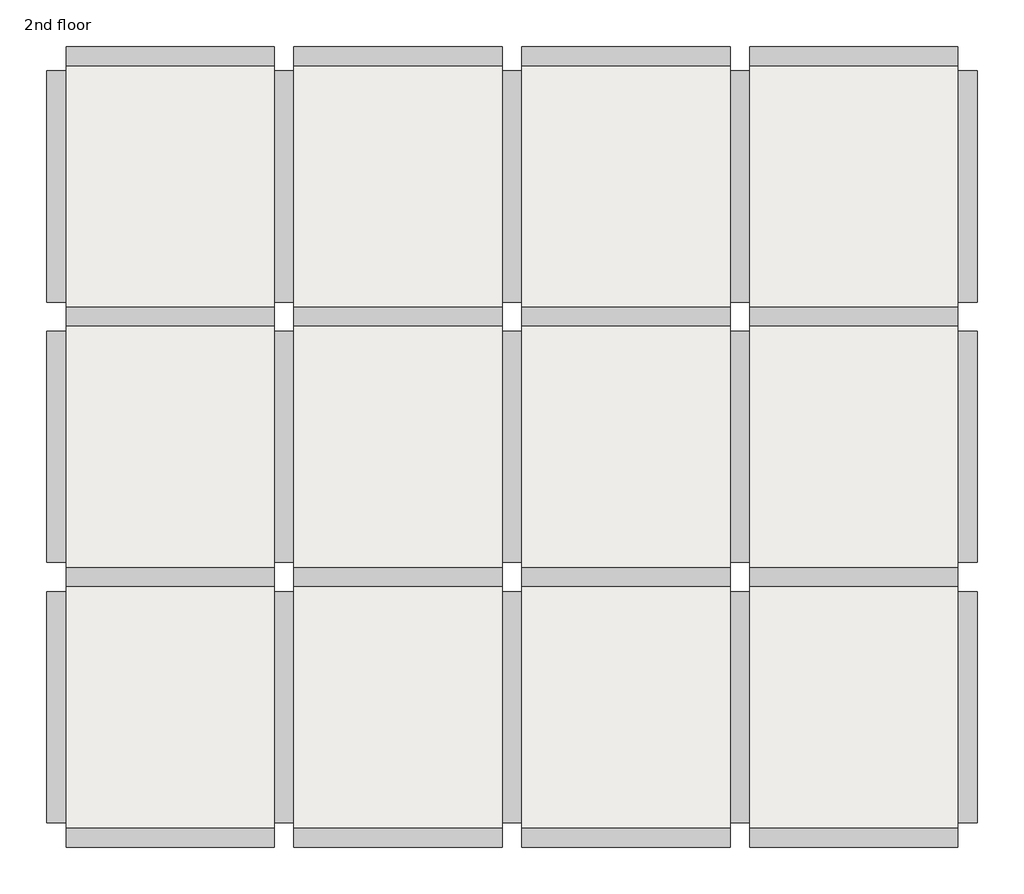
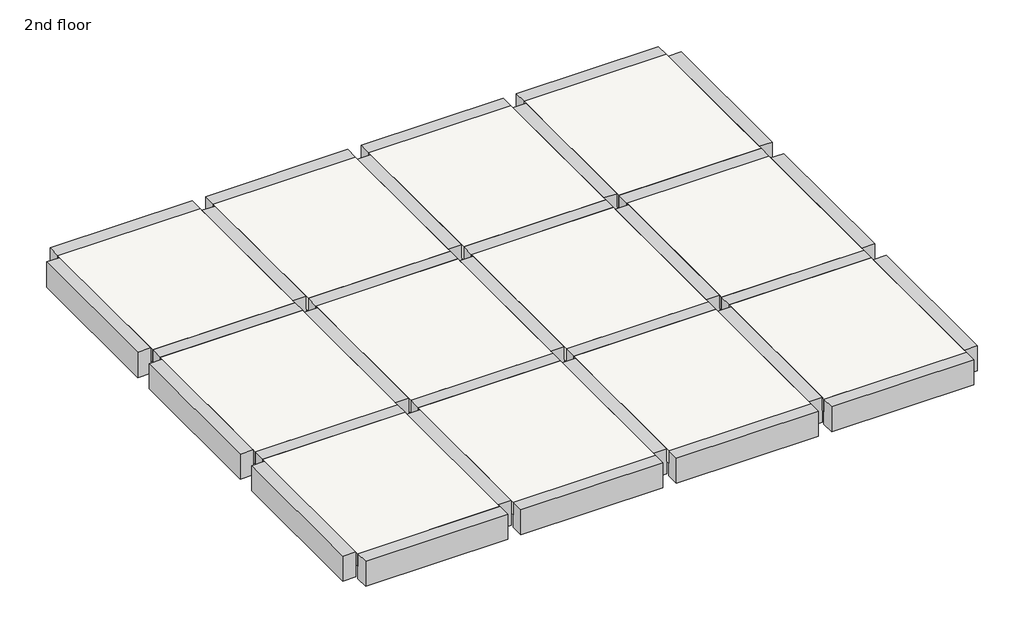
# One storey: 31 beams, 12 slabs.
"""IFC4 building model written with IfcOpenShell, lengths in millimetres."""

from ifc_helpers import new_model, si_unit, frame, origin, place, context, project, spatial, polyline, outline, extrude, faceted_brep, element, save

model = new_model("IFC4")

# Units and contexts
model_context = context("Model", 3, world=origin())
ifc_project = project(units=[si_unit("LENGTHUNIT", "METRE", prefix="MILLI")], contexts=[model_context])

# Site, building, storey
site = spatial("IfcSite", under=ifc_project)
building = spatial("IfcBuilding", under=site)
storey = spatial("IfcBuildingStorey", under=building, Name="2nd floor", Elevation=6096.0)

# Beams
placement = place(None, origin())
element("IfcBeam", 1, ObjectType="M_Concrete-Rectangular Beam : 300 x 600mm", at=placement, inside=storey, context=model_context, shape_type="SweptSolid", body=[
    extrude(outline(polyline([(-11389.0800189, 9311.4575251), (-11089.0800189, 9311.4575251), (-11089.0800189, 5761.4575251), (-11389.0800189, 5761.4575251), (-11389.0800189, 9311.4575251)])), frame((0.0, 0.0, 5496.0), z_axis=(0.0, 0.0, 1.0), x_axis=(1.0, 0.0, 0.0)), (0.0, 0.0, 1.0), 600.0),
])
element("IfcBeam", 2, ObjectType="M_Concrete-Rectangular Beam : 300 x 600mm", at=placement, inside=storey, context=model_context, shape_type="SweptSolid", body=[
    extrude(outline(polyline([(-11389.0800189, 13311.4575251), (-11089.0800189, 13311.4575251), (-11089.0800189, 9761.4575251), (-11389.0800189, 9761.4575251), (-11389.0800189, 13311.4575251)])), frame((0.0, 0.0, 5496.0), z_axis=(0.0, 0.0, 1.0), x_axis=(1.0, 0.0, 0.0)), (0.0, 0.0, 1.0), 600.0),
])
element("IfcBeam", 3, ObjectType="M_Concrete-Rectangular Beam : 300 x 600mm", at=placement, inside=storey, context=model_context, shape_type="SweptSolid", body=[
    extrude(outline(polyline([(-11389.0800189, 17311.4575251), (-11089.0800189, 17311.4575251), (-11089.0800189, 13761.4575251), (-11389.0800189, 13761.4575251), (-11389.0800189, 17311.4575251)])), frame((0.0, 0.0, 5496.0), z_axis=(0.0, 0.0, 1.0), x_axis=(1.0, 0.0, 0.0)), (0.0, 0.0, 1.0), 600.0),
])
element("IfcBeam", 4, ObjectType="M_Concrete-Rectangular Beam : 300 x 600mm", at=placement, inside=storey, context=model_context, shape_type="SweptSolid", body=[
    extrude(outline(polyline([(-7889.0800189, 9311.4575251), (-7589.0800189, 9311.4575251), (-7589.0800189, 5761.4575251), (-7889.0800189, 5761.4575251), (-7889.0800189, 9311.4575251)])), frame((0.0, 0.0, 5496.0), z_axis=(0.0, 0.0, 1.0), x_axis=(1.0, 0.0, 0.0)), (0.0, 0.0, 1.0), 600.0),
])
element("IfcBeam", 5, ObjectType="M_Concrete-Rectangular Beam : 300 x 600mm", at=placement, inside=storey, context=model_context, shape_type="SweptSolid", body=[
    extrude(outline(polyline([(-7889.0800189, 13311.4575251), (-7589.0800189, 13311.4575251), (-7589.0800189, 9761.4575251), (-7889.0800189, 9761.4575251), (-7889.0800189, 13311.4575251)])), frame((0.0, 0.0, 5496.0), z_axis=(0.0, 0.0, 1.0), x_axis=(1.0, 0.0, 0.0)), (0.0, 0.0, 1.0), 600.0),
])
element("IfcBeam", 6, ObjectType="M_Concrete-Rectangular Beam : 300 x 600mm", at=placement, inside=storey, context=model_context, shape_type="SweptSolid", body=[
    extrude(outline(polyline([(-7889.0800189, 17311.4575251), (-7589.0800189, 17311.4575251), (-7589.0800189, 13761.4575251), (-7889.0800189, 13761.4575251), (-7889.0800189, 17311.4575251)])), frame((0.0, 0.0, 5496.0), z_axis=(0.0, 0.0, 1.0), x_axis=(1.0, 0.0, 0.0)), (0.0, 0.0, 1.0), 600.0),
])
element("IfcBeam", 7, ObjectType="M_Concrete-Rectangular Beam : 300 x 600mm", at=placement, inside=storey, context=model_context, shape_type="SweptSolid", body=[
    extrude(outline(polyline([(-4389.0800189, 9311.4575251), (-4089.0800189, 9311.4575251), (-4089.0800189, 5761.4575251), (-4389.0800189, 5761.4575251), (-4389.0800189, 9311.4575251)])), frame((0.0, 0.0, 5496.0), z_axis=(0.0, 0.0, 1.0), x_axis=(1.0, 0.0, 0.0)), (0.0, 0.0, 1.0), 600.0),
])
element("IfcBeam", 8, ObjectType="M_Concrete-Rectangular Beam : 300 x 600mm", at=placement, inside=storey, context=model_context, shape_type="SweptSolid", body=[
    extrude(outline(polyline([(-4389.0800189, 13311.4575251), (-4089.0800189, 13311.4575251), (-4089.0800189, 9761.4575251), (-4389.0800189, 9761.4575251), (-4389.0800189, 13311.4575251)])), frame((0.0, 0.0, 5496.0), z_axis=(0.0, 0.0, 1.0), x_axis=(1.0, 0.0, 0.0)), (0.0, 0.0, 1.0), 600.0),
])
element("IfcBeam", 9, ObjectType="M_Concrete-Rectangular Beam : 300 x 600mm", at=placement, inside=storey, context=model_context, shape_type="SweptSolid", body=[
    extrude(outline(polyline([(-4389.0800189, 17311.4575251), (-4089.0800189, 17311.4575251), (-4089.0800189, 13761.4575251), (-4389.0800189, 13761.4575251), (-4389.0800189, 17311.4575251)])), frame((0.0, 0.0, 5496.0), z_axis=(0.0, 0.0, 1.0), x_axis=(1.0, 0.0, 0.0)), (0.0, 0.0, 1.0), 600.0),
])
element("IfcBeam", 10, ObjectType="M_Concrete-Rectangular Beam : 300 x 600mm", at=placement, inside=storey, context=model_context, shape_type="SweptSolid", body=[
    extrude(outline(polyline([(-889.0800189, 9311.4575251), (-589.0800189, 9311.4575251), (-589.0800189, 5761.4575251), (-889.0800189, 5761.4575251), (-889.0800189, 9311.4575251)])), frame((0.0, 0.0, 5496.0), z_axis=(0.0, 0.0, 1.0), x_axis=(1.0, 0.0, 0.0)), (0.0, 0.0, 1.0), 600.0),
])
element("IfcBeam", 11, ObjectType="M_Concrete-Rectangular Beam : 300 x 600mm", at=placement, inside=storey, context=model_context, shape_type="SweptSolid", body=[
    extrude(outline(polyline([(-889.0800189, 13311.4575251), (-589.0800189, 13311.4575251), (-589.0800189, 9761.4575251), (-889.0800189, 9761.4575251), (-889.0800189, 13311.4575251)])), frame((0.0, 0.0, 5496.0), z_axis=(0.0, 0.0, 1.0), x_axis=(1.0, 0.0, 0.0)), (0.0, 0.0, 1.0), 600.0),
])
element("IfcBeam", 12, ObjectType="M_Concrete-Rectangular Beam : 300 x 600mm", at=placement, inside=storey, context=model_context, shape_type="SweptSolid", body=[
    extrude(outline(polyline([(-889.0800189, 17311.4575251), (-589.0800189, 17311.4575251), (-589.0800189, 13761.4575251), (-889.0800189, 13761.4575251), (-889.0800189, 17311.4575251)])), frame((0.0, 0.0, 5496.0), z_axis=(0.0, 0.0, 1.0), x_axis=(1.0, 0.0, 0.0)), (0.0, 0.0, 1.0), 600.0),
])
element("IfcBeam", 13, ObjectType="M_Concrete-Rectangular Beam : 300 x 600mm", at=placement, inside=storey, context=model_context, shape_type="SweptSolid", body=[
    extrude(outline(polyline([(2610.9199811, 9311.4575251), (2910.9199811, 9311.4575251), (2910.9199811, 5761.4575251), (2610.9199811, 5761.4575251), (2610.9199811, 9311.4575251)])), frame((0.0, 0.0, 5496.0), z_axis=(0.0, 0.0, 1.0), x_axis=(1.0, 0.0, 0.0)), (0.0, 0.0, 1.0), 600.0),
])
element("IfcBeam", 14, ObjectType="M_Concrete-Rectangular Beam : 300 x 600mm", at=placement, inside=storey, context=model_context, shape_type="SweptSolid", body=[
    extrude(outline(polyline([(2610.9199811, 13311.4575251), (2910.9199811, 13311.4575251), (2910.9199811, 9761.4575251), (2610.9199811, 9761.4575251), (2610.9199811, 13311.4575251)])), frame((0.0, 0.0, 5496.0), z_axis=(0.0, 0.0, 1.0), x_axis=(1.0, 0.0, 0.0)), (0.0, 0.0, 1.0), 600.0),
])
element("IfcBeam", 15, ObjectType="M_Concrete-Rectangular Beam : 300 x 600mm", at=placement, inside=storey, context=model_context, shape_type="SweptSolid", body=[
    extrude(outline(polyline([(2610.9199811, 17311.4575251), (2910.9199811, 17311.4575251), (2910.9199811, 13761.4575251), (2610.9199811, 13761.4575251), (2610.9199811, 17311.4575251)])), frame((0.0, 0.0, 5496.0), z_axis=(0.0, 0.0, 1.0), x_axis=(1.0, 0.0, 0.0)), (0.0, 0.0, 1.0), 600.0),
])
element("IfcBeam", 16, ObjectType="M_Concrete-Rectangular Beam : 300 x 600mm", at=placement, inside=storey, context=model_context, shape_type="Brep", body=[
    faceted_brep([(-11089.0800189, 17386.4575251, 6096.0), (-7889.0800189, 17386.4575251, 6096.0), (-7889.0800189, 17686.4575251, 6096.0), (-11089.0800189, 17686.4575251, 6096.0), (-11089.0800189, 17386.4575251, 5796.0), (-11089.0800189, 17386.4575251, 5496.0), (-7889.0800189, 17386.4575251, 5496.0), (-7889.0800189, 17386.4575251, 5796.0), (-7889.0800189, 17686.4575251, 5496.0), (-11089.0800189, 17686.4575251, 5496.0)], [[[0, 1, 2, 3]], [[0, 4, 5, 6, 7, 1]], [[8, 6, 5, 9]], [[9, 3, 2, 8]], [[5, 4, 0, 3, 9]], [[1, 7, 6, 8, 2]]]),
])
element("IfcBeam", 17, ObjectType="M_Concrete-Rectangular Beam : 300 x 600mm", at=placement, inside=storey, context=model_context, shape_type="Brep", body=[
    faceted_brep([(-7589.0800189, 17386.4575251, 6096.0), (-4389.0800189, 17386.4575251, 6096.0), (-4389.0800189, 17686.4575251, 6096.0), (-7589.0800189, 17686.4575251, 6096.0), (-7589.0800189, 17386.4575251, 5796.0), (-7589.0800189, 17386.4575251, 5496.0), (-4389.0800189, 17386.4575251, 5496.0), (-4389.0800189, 17386.4575251, 5796.0), (-4389.0800189, 17686.4575251, 5496.0), (-7589.0800189, 17686.4575251, 5496.0)], [[[0, 1, 2, 3]], [[0, 4, 5, 6, 7, 1]], [[8, 6, 5, 9]], [[9, 3, 2, 8]], [[5, 4, 0, 3, 9]], [[1, 7, 6, 8, 2]]]),
])
element("IfcBeam", 18, ObjectType="M_Concrete-Rectangular Beam : 300 x 600mm", at=placement, inside=storey, context=model_context, shape_type="Brep", body=[
    faceted_brep([(-4089.0800189, 17386.4575251, 6096.0), (-889.0800189, 17386.4575251, 6096.0), (-889.0800189, 17686.4575251, 6096.0), (-4089.0800189, 17686.4575251, 6096.0), (-4089.0800189, 17386.4575251, 5796.0), (-4089.0800189, 17386.4575251, 5496.0), (-889.0800189, 17386.4575251, 5496.0), (-889.0800189, 17386.4575251, 5796.0), (-889.0800189, 17686.4575251, 5496.0), (-4089.0800189, 17686.4575251, 5496.0)], [[[0, 1, 2, 3]], [[0, 4, 5, 6, 7, 1]], [[8, 6, 5, 9]], [[9, 3, 2, 8]], [[5, 4, 0, 3, 9]], [[1, 7, 6, 8, 2]]]),
])
element("IfcBeam", 19, ObjectType="M_Concrete-Rectangular Beam : 300 x 600mm", at=placement, inside=storey, context=model_context, shape_type="Brep", body=[
    faceted_brep([(-589.0800189, 17386.4575251, 6096.0), (2610.9199811, 17386.4575251, 6096.0), (2610.9199811, 17686.4575251, 6096.0), (-589.0800189, 17686.4575251, 6096.0), (-589.0800189, 17386.4575251, 5796.0), (-589.0800189, 17386.4575251, 5496.0), (2610.9199811, 17386.4575251, 5496.0), (2610.9199811, 17386.4575251, 5796.0), (2610.9199811, 17686.4575251, 5496.0), (-589.0800189, 17686.4575251, 5496.0)], [[[0, 1, 2, 3]], [[0, 4, 5, 6, 7, 1]], [[8, 6, 5, 9]], [[9, 3, 2, 8]], [[5, 4, 0, 3, 9]], [[1, 7, 6, 8, 2]]]),
])
element("IfcBeam", 20, ObjectType="M_Concrete-Rectangular Beam : 300 x 600mm", at=placement, inside=storey, context=model_context, shape_type="Brep", body=[
    faceted_brep([(-11089.0800189, 13386.4575251, 6096.0), (-7889.0800189, 13386.4575251, 6096.0), (-7889.0800189, 13686.4575251, 6096.0), (-11089.0800189, 13686.4575251, 6096.0), (-11089.0800189, 13386.4575251, 5796.0), (-11089.0800189, 13386.4575251, 5496.0), (-7889.0800189, 13386.4575251, 5496.0), (-7889.0800189, 13386.4575251, 5796.0), (-7889.0800189, 13686.4575251, 5496.0), (-11089.0800189, 13686.4575251, 5496.0), (-11089.0800189, 13686.4575251, 5796.0), (-7889.0800189, 13686.4575251, 5796.0)], [[[0, 1, 2, 3]], [[0, 4, 5, 6, 7, 1]], [[8, 6, 5, 9]], [[9, 10, 3, 2, 11, 8]], [[5, 4, 0, 3, 10, 9]], [[1, 7, 6, 8, 11, 2]]]),
])
element("IfcBeam", 21, ObjectType="M_Concrete-Rectangular Beam : 300 x 600mm", at=placement, inside=storey, context=model_context, shape_type="Brep", body=[
    faceted_brep([(-7589.0800189, 13686.4575251, 6096.0), (-7589.0800189, 13386.4575251, 6096.0), (-4389.0800189, 13386.4575251, 6096.0), (-4389.0800189, 13686.4575251, 6096.0), (-7589.0800189, 13386.4575251, 5796.0), (-7589.0800189, 13386.4575251, 5496.0), (-4389.0800189, 13386.4575251, 5496.0), (-4389.0800189, 13386.4575251, 5796.0), (-7589.0800189, 13686.4575251, 5496.0), (-4389.0800189, 13686.4575251, 5496.0), (-7589.0800189, 13686.4575251, 5796.0), (-4389.0800189, 13686.4575251, 5796.0)], [[[0, 1, 2, 3]], [[1, 4, 5, 6, 7, 2]], [[5, 8, 9, 6]], [[8, 10, 0, 3, 11, 9]], [[5, 4, 1, 0, 10, 8]], [[2, 7, 6, 9, 11, 3]]]),
])
element("IfcBeam", 22, ObjectType="M_Concrete-Rectangular Beam : 300 x 600mm", at=placement, inside=storey, context=model_context, shape_type="Brep", body=[
    faceted_brep([(-4089.0800189, 13686.4575251, 6096.0), (-4089.0800189, 13386.4575251, 6096.0), (-889.0800189, 13386.4575251, 6096.0), (-889.0800189, 13686.4575251, 6096.0), (-4089.0800189, 13386.4575251, 5796.0), (-4089.0800189, 13386.4575251, 5496.0), (-889.0800189, 13386.4575251, 5496.0), (-889.0800189, 13386.4575251, 5796.0), (-4089.0800189, 13686.4575251, 5496.0), (-889.0800189, 13686.4575251, 5496.0), (-4089.0800189, 13686.4575251, 5796.0), (-889.0800189, 13686.4575251, 5796.0)], [[[0, 1, 2, 3]], [[1, 4, 5, 6, 7, 2]], [[5, 8, 9, 6]], [[8, 10, 0, 3, 11, 9]], [[5, 4, 1, 0, 10, 8]], [[2, 7, 6, 9, 11, 3]]]),
])
element("IfcBeam", 23, ObjectType="M_Concrete-Rectangular Beam : 300 x 600mm", at=placement, inside=storey, context=model_context, shape_type="Brep", body=[
    faceted_brep([(-589.0800189, 13686.4575251, 6096.0), (-589.0800189, 13386.4575251, 6096.0), (2610.9199811, 13386.4575251, 6096.0), (2610.9199811, 13686.4575251, 6096.0), (-589.0800189, 13386.4575251, 5796.0), (-589.0800189, 13386.4575251, 5496.0), (2610.9199811, 13386.4575251, 5496.0), (2610.9199811, 13386.4575251, 5796.0), (-589.0800189, 13686.4575251, 5496.0), (2610.9199811, 13686.4575251, 5496.0), (-589.0800189, 13686.4575251, 5796.0), (2610.9199811, 13686.4575251, 5796.0)], [[[0, 1, 2, 3]], [[1, 4, 5, 6, 7, 2]], [[5, 8, 9, 6]], [[8, 10, 0, 3, 11, 9]], [[5, 4, 1, 0, 10, 8]], [[2, 7, 6, 9, 11, 3]]]),
])
element("IfcBeam", 24, ObjectType="M_Concrete-Rectangular Beam : 300 x 600mm", at=placement, inside=storey, context=model_context, shape_type="Brep", body=[
    faceted_brep([(-11089.0800189, 9386.4575251, 6096.0), (-7889.0800189, 9386.4575251, 6096.0), (-7889.0800189, 9686.4575251, 6096.0), (-11089.0800189, 9686.4575251, 6096.0), (-11089.0800189, 9386.4575251, 5796.0), (-11089.0800189, 9386.4575251, 5496.0), (-7889.0800189, 9386.4575251, 5496.0), (-7889.0800189, 9386.4575251, 5796.0), (-7889.0800189, 9686.4575251, 5496.0), (-11089.0800189, 9686.4575251, 5496.0), (-11089.0800189, 9686.4575251, 5796.0), (-7889.0800189, 9686.4575251, 5796.0)], [[[0, 1, 2, 3]], [[0, 4, 5, 6, 7, 1]], [[8, 6, 5, 9]], [[9, 10, 3, 2, 11, 8]], [[5, 4, 0, 3, 10, 9]], [[1, 7, 6, 8, 11, 2]]]),
])
element("IfcBeam", 25, ObjectType="M_Concrete-Rectangular Beam : 300 x 600mm", at=placement, inside=storey, context=model_context, shape_type="Brep", body=[
    faceted_brep([(-7589.0800189, 9686.4575251, 6096.0), (-7589.0800189, 9386.4575251, 6096.0), (-4389.0800189, 9386.4575251, 6096.0), (-4389.0800189, 9686.4575251, 6096.0), (-7589.0800189, 9386.4575251, 5796.0), (-7589.0800189, 9386.4575251, 5496.0), (-4389.0800189, 9386.4575251, 5496.0), (-4389.0800189, 9386.4575251, 5796.0), (-7589.0800189, 9686.4575251, 5496.0), (-4389.0800189, 9686.4575251, 5496.0), (-7589.0800189, 9686.4575251, 5796.0), (-4389.0800189, 9686.4575251, 5796.0)], [[[0, 1, 2, 3]], [[1, 4, 5, 6, 7, 2]], [[5, 8, 9, 6]], [[8, 10, 0, 3, 11, 9]], [[5, 4, 1, 0, 10, 8]], [[2, 7, 6, 9, 11, 3]]]),
])
element("IfcBeam", 26, ObjectType="M_Concrete-Rectangular Beam : 300 x 600mm", at=placement, inside=storey, context=model_context, shape_type="Brep", body=[
    faceted_brep([(-4089.0800189, 9686.4575251, 6096.0), (-4089.0800189, 9386.4575251, 6096.0), (-889.0800189, 9386.4575251, 6096.0), (-889.0800189, 9686.4575251, 6096.0), (-4089.0800189, 9386.4575251, 5796.0), (-4089.0800189, 9386.4575251, 5496.0), (-889.0800189, 9386.4575251, 5496.0), (-889.0800189, 9386.4575251, 5796.0), (-4089.0800189, 9686.4575251, 5496.0), (-889.0800189, 9686.4575251, 5496.0), (-4089.0800189, 9686.4575251, 5796.0), (-889.0800189, 9686.4575251, 5796.0)], [[[0, 1, 2, 3]], [[1, 4, 5, 6, 7, 2]], [[5, 8, 9, 6]], [[8, 10, 0, 3, 11, 9]], [[5, 4, 1, 0, 10, 8]], [[2, 7, 6, 9, 11, 3]]]),
])
element("IfcBeam", 27, ObjectType="M_Concrete-Rectangular Beam : 300 x 600mm", at=placement, inside=storey, context=model_context, shape_type="Brep", body=[
    faceted_brep([(-589.0800189, 9686.4575251, 6096.0), (-589.0800189, 9386.4575251, 6096.0), (2610.9199811, 9386.4575251, 6096.0), (2610.9199811, 9686.4575251, 6096.0), (-589.0800189, 9386.4575251, 5796.0), (-589.0800189, 9386.4575251, 5496.0), (2610.9199811, 9386.4575251, 5496.0), (2610.9199811, 9386.4575251, 5796.0), (-589.0800189, 9686.4575251, 5496.0), (2610.9199811, 9686.4575251, 5496.0), (-589.0800189, 9686.4575251, 5796.0), (2610.9199811, 9686.4575251, 5796.0)], [[[0, 1, 2, 3]], [[1, 4, 5, 6, 7, 2]], [[5, 8, 9, 6]], [[8, 10, 0, 3, 11, 9]], [[5, 4, 1, 0, 10, 8]], [[2, 7, 6, 9, 11, 3]]]),
])
element("IfcBeam", 28, ObjectType="M_Concrete-Rectangular Beam : 300 x 600mm", at=placement, inside=storey, context=model_context, shape_type="Brep", body=[
    faceted_brep([(-7889.0800189, 5386.4575251, 6096.0), (-7889.0800189, 5686.4575251, 6096.0), (-11089.0800189, 5686.4575251, 6096.0), (-11089.0800189, 5386.4575251, 6096.0), (-11089.0800189, 5386.4575251, 5496.0), (-7889.0800189, 5386.4575251, 5496.0), (-11089.0800189, 5686.4575251, 5496.0), (-7889.0800189, 5686.4575251, 5496.0), (-11089.0800189, 5686.4575251, 5796.0), (-7889.0800189, 5686.4575251, 5796.0)], [[[0, 1, 2, 3]], [[3, 4, 5, 0]], [[6, 7, 5, 4]], [[6, 8, 2, 1, 9, 7]], [[2, 8, 6, 4, 3]], [[0, 5, 7, 9, 1]]]),
])
element("IfcBeam", 29, ObjectType="M_Concrete-Rectangular Beam : 300 x 600mm", at=placement, inside=storey, context=model_context, shape_type="Brep", body=[
    faceted_brep([(-4389.0800189, 5386.4575251, 6096.0), (-4389.0800189, 5686.4575251, 6096.0), (-7589.0800189, 5686.4575251, 6096.0), (-7589.0800189, 5386.4575251, 6096.0), (-7589.0800189, 5386.4575251, 5496.0), (-4389.0800189, 5386.4575251, 5496.0), (-7589.0800189, 5686.4575251, 5496.0), (-4389.0800189, 5686.4575251, 5496.0), (-7589.0800189, 5686.4575251, 5796.0), (-4389.0800189, 5686.4575251, 5796.0)], [[[0, 1, 2, 3]], [[3, 4, 5, 0]], [[6, 7, 5, 4]], [[6, 8, 2, 1, 9, 7]], [[2, 8, 6, 4, 3]], [[0, 5, 7, 9, 1]]]),
])
element("IfcBeam", 30, ObjectType="M_Concrete-Rectangular Beam : 300 x 600mm", at=placement, inside=storey, context=model_context, shape_type="Brep", body=[
    faceted_brep([(-889.0800189, 5386.4575251, 6096.0), (-889.0800189, 5686.4575251, 6096.0), (-4089.0800189, 5686.4575251, 6096.0), (-4089.0800189, 5386.4575251, 6096.0), (-4089.0800189, 5386.4575251, 5496.0), (-889.0800189, 5386.4575251, 5496.0), (-4089.0800189, 5686.4575251, 5496.0), (-889.0800189, 5686.4575251, 5496.0), (-4089.0800189, 5686.4575251, 5796.0), (-889.0800189, 5686.4575251, 5796.0)], [[[0, 1, 2, 3]], [[3, 4, 5, 0]], [[6, 7, 5, 4]], [[6, 8, 2, 1, 9, 7]], [[2, 8, 6, 4, 3]], [[0, 5, 7, 9, 1]]]),
])
element("IfcBeam", 31, ObjectType="M_Concrete-Rectangular Beam : 300 x 600mm", at=placement, inside=storey, context=model_context, shape_type="Brep", body=[
    faceted_brep([(2610.9199811, 5386.4575251, 6096.0), (2610.9199811, 5686.4575251, 6096.0), (-589.0800189, 5686.4575251, 6096.0), (-589.0800189, 5386.4575251, 6096.0), (-589.0800189, 5386.4575251, 5496.0), (2610.9199811, 5386.4575251, 5496.0), (-589.0800189, 5686.4575251, 5496.0), (2610.9199811, 5686.4575251, 5496.0), (-589.0800189, 5686.4575251, 5796.0), (2610.9199811, 5686.4575251, 5796.0)], [[[0, 1, 2, 3]], [[3, 4, 5, 0]], [[6, 7, 5, 4]], [[6, 8, 2, 1, 9, 7]], [[2, 8, 6, 4, 3]], [[0, 5, 7, 9, 1]]]),
])

# Slabs
element("IfcSlab", 32, ObjectType="Generic 300mm", at=placement, inside=storey, context=model_context, shape_type="Brep", body=[
    faceted_brep([(-7889.0800189, 17386.4575251, 5796.0), (-7889.0800189, 13686.4575251, 5796.0), (-11089.0800189, 13686.4575251, 5796.0), (-11089.0800189, 17386.4575251, 5796.0), (-7889.0800189, 17386.4575251, 6096.0), (-11089.0800189, 17386.4575251, 6096.0), (-11089.0800189, 17311.4575251, 6096.0), (-11089.0800189, 13761.4575251, 6096.0), (-11089.0800189, 13686.4575251, 6096.0), (-7889.0800189, 13686.4575251, 6096.0), (-7889.0800189, 13761.4575251, 6096.0), (-7889.0800189, 17311.4575251, 6096.0)], [[[0, 1, 2, 3]], [[4, 5, 6, 7, 8, 9, 10, 11]], [[1, 0, 4, 11, 10, 9]], [[2, 1, 9, 8]], [[3, 2, 8, 7, 6, 5]], [[0, 3, 5, 4]]]),
])
element("IfcSlab", 33, ObjectType="Generic 300mm", at=placement, inside=storey, context=model_context, shape_type="Brep", body=[
    faceted_brep([(-4389.0800189, 17386.4575251, 5796.0), (-4389.0800189, 13686.4575251, 5796.0), (-7589.0800189, 13686.4575251, 5796.0), (-7589.0800189, 17386.4575251, 5796.0), (-4389.0800189, 17386.4575251, 6096.0), (-7589.0800189, 17386.4575251, 6096.0), (-7589.0800189, 17311.4575251, 6096.0), (-7589.0800189, 13761.4575251, 6096.0), (-7589.0800189, 13686.4575251, 6096.0), (-4389.0800189, 13686.4575251, 6096.0), (-4389.0800189, 13761.4575251, 6096.0), (-4389.0800189, 17311.4575251, 6096.0)], [[[0, 1, 2, 3]], [[4, 5, 6, 7, 8, 9, 10, 11]], [[1, 0, 4, 11, 10, 9]], [[2, 1, 9, 8]], [[3, 2, 8, 7, 6, 5]], [[0, 3, 5, 4]]]),
])
element("IfcSlab", 34, ObjectType="Generic 300mm", at=placement, inside=storey, context=model_context, shape_type="Brep", body=[
    faceted_brep([(-889.0800189, 17386.4575251, 5796.0), (-889.0800189, 13686.4575251, 5796.0), (-4089.0800189, 13686.4575251, 5796.0), (-4089.0800189, 17386.4575251, 5796.0), (-889.0800189, 17386.4575251, 6096.0), (-4089.0800189, 17386.4575251, 6096.0), (-4089.0800189, 17311.4575251, 6096.0), (-4089.0800189, 13761.4575251, 6096.0), (-4089.0800189, 13686.4575251, 6096.0), (-889.0800189, 13686.4575251, 6096.0), (-889.0800189, 13761.4575251, 6096.0), (-889.0800189, 17311.4575251, 6096.0)], [[[0, 1, 2, 3]], [[4, 5, 6, 7, 8, 9, 10, 11]], [[1, 0, 4, 11, 10, 9]], [[2, 1, 9, 8]], [[3, 2, 8, 7, 6, 5]], [[0, 3, 5, 4]]]),
])
element("IfcSlab", 35, ObjectType="Generic 300mm", at=placement, inside=storey, context=model_context, shape_type="Brep", body=[
    faceted_brep([(2610.9199811, 17386.4575251, 5796.0), (2610.9199811, 13686.4575251, 5796.0), (-589.0800189, 13686.4575251, 5796.0), (-589.0800189, 17386.4575251, 5796.0), (2610.9199811, 17386.4575251, 6096.0), (-589.0800189, 17386.4575251, 6096.0), (-589.0800189, 17311.4575251, 6096.0), (-589.0800189, 13761.4575251, 6096.0), (-589.0800189, 13686.4575251, 6096.0), (2610.9199811, 13686.4575251, 6096.0), (2610.9199811, 13761.4575251, 6096.0), (2610.9199811, 17311.4575251, 6096.0)], [[[0, 1, 2, 3]], [[4, 5, 6, 7, 8, 9, 10, 11]], [[1, 0, 4, 11, 10, 9]], [[2, 1, 9, 8]], [[3, 2, 8, 7, 6, 5]], [[0, 3, 5, 4]]]),
])
element("IfcSlab", 36, ObjectType="Generic 300mm", at=placement, inside=storey, context=model_context, shape_type="Brep", body=[
    faceted_brep([(2610.9199811, 13386.4575251, 5796.0), (2610.9199811, 9686.4575251, 5796.0), (-589.0800189, 9686.4575251, 5796.0), (-589.0800189, 13386.4575251, 5796.0), (2610.9199811, 13386.4575251, 6096.0), (-589.0800189, 13386.4575251, 6096.0), (-589.0800189, 13311.4575251, 6096.0), (-589.0800189, 9761.4575251, 6096.0), (-589.0800189, 9686.4575251, 6096.0), (2610.9199811, 9686.4575251, 6096.0), (2610.9199811, 9761.4575251, 6096.0), (2610.9199811, 13311.4575251, 6096.0)], [[[0, 1, 2, 3]], [[4, 5, 6, 7, 8, 9, 10, 11]], [[1, 0, 4, 11, 10, 9]], [[2, 1, 9, 8]], [[3, 2, 8, 7, 6, 5]], [[0, 3, 5, 4]]]),
])
element("IfcSlab", 37, ObjectType="Generic 300mm", at=placement, inside=storey, context=model_context, shape_type="Brep", body=[
    faceted_brep([(2610.9199811, 9386.4575251, 5796.0), (2610.9199811, 5686.4575251, 5796.0), (-589.0800189, 5686.4575251, 5796.0), (-589.0800189, 9386.4575251, 5796.0), (2610.9199811, 9386.4575251, 6096.0), (-589.0800189, 9386.4575251, 6096.0), (-589.0800189, 9311.4575251, 6096.0), (-589.0800189, 5761.4575251, 6096.0), (-589.0800189, 5686.4575251, 6096.0), (2610.9199811, 5686.4575251, 6096.0), (2610.9199811, 5761.4575251, 6096.0), (2610.9199811, 9311.4575251, 6096.0)], [[[0, 1, 2, 3]], [[4, 5, 6, 7, 8, 9, 10, 11]], [[1, 0, 4, 11, 10, 9]], [[2, 1, 9, 8]], [[3, 2, 8, 7, 6, 5]], [[0, 3, 5, 4]]]),
])
element("IfcSlab", 38, ObjectType="Generic 300mm", at=placement, inside=storey, context=model_context, shape_type="Brep", body=[
    faceted_brep([(-889.0800189, 9386.4575251, 5796.0), (-889.0800189, 5686.4575251, 5796.0), (-4089.0800189, 5686.4575251, 5796.0), (-4089.0800189, 9386.4575251, 5796.0), (-889.0800189, 9386.4575251, 6096.0), (-4089.0800189, 9386.4575251, 6096.0), (-4089.0800189, 9311.4575251, 6096.0), (-4089.0800189, 5761.4575251, 6096.0), (-4089.0800189, 5686.4575251, 6096.0), (-889.0800189, 5686.4575251, 6096.0), (-889.0800189, 5761.4575251, 6096.0), (-889.0800189, 9311.4575251, 6096.0)], [[[0, 1, 2, 3]], [[4, 5, 6, 7, 8, 9, 10, 11]], [[1, 0, 4, 11, 10, 9]], [[2, 1, 9, 8]], [[3, 2, 8, 7, 6, 5]], [[0, 3, 5, 4]]]),
])
element("IfcSlab", 39, ObjectType="Generic 300mm", at=placement, inside=storey, context=model_context, shape_type="Brep", body=[
    faceted_brep([(-4389.0800189, 9386.4575251, 5796.0), (-4389.0800189, 5686.4575251, 5796.0), (-7589.0800189, 5686.4575251, 5796.0), (-7589.0800189, 9386.4575251, 5796.0), (-4389.0800189, 9386.4575251, 6096.0), (-7589.0800189, 9386.4575251, 6096.0), (-7589.0800189, 9311.4575251, 6096.0), (-7589.0800189, 5761.4575251, 6096.0), (-7589.0800189, 5686.4575251, 6096.0), (-4389.0800189, 5686.4575251, 6096.0), (-4389.0800189, 5761.4575251, 6096.0), (-4389.0800189, 9311.4575251, 6096.0)], [[[0, 1, 2, 3]], [[4, 5, 6, 7, 8, 9, 10, 11]], [[1, 0, 4, 11, 10, 9]], [[2, 1, 9, 8]], [[3, 2, 8, 7, 6, 5]], [[0, 3, 5, 4]]]),
])
element("IfcSlab", 40, ObjectType="Generic 300mm", at=placement, inside=storey, context=model_context, shape_type="Brep", body=[
    faceted_brep([(-7889.0800189, 9386.4575251, 5796.0), (-7889.0800189, 5686.4575251, 5796.0), (-11089.0800189, 5686.4575251, 5796.0), (-11089.0800189, 9386.4575251, 5796.0), (-7889.0800189, 9386.4575251, 6096.0), (-11089.0800189, 9386.4575251, 6096.0), (-11089.0800189, 9311.4575251, 6096.0), (-11089.0800189, 5761.4575251, 6096.0), (-11089.0800189, 5686.4575251, 6096.0), (-7889.0800189, 5686.4575251, 6096.0), (-7889.0800189, 5761.4575251, 6096.0), (-7889.0800189, 9311.4575251, 6096.0)], [[[0, 1, 2, 3]], [[4, 5, 6, 7, 8, 9, 10, 11]], [[1, 0, 4, 11, 10, 9]], [[2, 1, 9, 8]], [[3, 2, 8, 7, 6, 5]], [[0, 3, 5, 4]]]),
])
element("IfcSlab", 41, ObjectType="Generic 300mm", at=placement, inside=storey, context=model_context, shape_type="Brep", body=[
    faceted_brep([(-7889.0800189, 13386.4575251, 5796.0), (-7889.0800189, 9686.4575251, 5796.0), (-11089.0800189, 9686.4575251, 5796.0), (-11089.0800189, 13386.4575251, 5796.0), (-7889.0800189, 13386.4575251, 6096.0), (-11089.0800189, 13386.4575251, 6096.0), (-11089.0800189, 13311.4575251, 6096.0), (-11089.0800189, 9761.4575251, 6096.0), (-11089.0800189, 9686.4575251, 6096.0), (-7889.0800189, 9686.4575251, 6096.0), (-7889.0800189, 9761.4575251, 6096.0), (-7889.0800189, 13311.4575251, 6096.0)], [[[0, 1, 2, 3]], [[4, 5, 6, 7, 8, 9, 10, 11]], [[1, 0, 4, 11, 10, 9]], [[2, 1, 9, 8]], [[3, 2, 8, 7, 6, 5]], [[0, 3, 5, 4]]]),
])
element("IfcSlab", 42, ObjectType="Generic 300mm", at=placement, inside=storey, context=model_context, shape_type="Brep", body=[
    faceted_brep([(-4389.0800189, 13386.4575251, 5796.0), (-4389.0800189, 9686.4575251, 5796.0), (-7589.0800189, 9686.4575251, 5796.0), (-7589.0800189, 13386.4575251, 5796.0), (-4389.0800189, 13386.4575251, 6096.0), (-7589.0800189, 13386.4575251, 6096.0), (-7589.0800189, 13311.4575251, 6096.0), (-7589.0800189, 9761.4575251, 6096.0), (-7589.0800189, 9686.4575251, 6096.0), (-4389.0800189, 9686.4575251, 6096.0), (-4389.0800189, 9761.4575251, 6096.0), (-4389.0800189, 13311.4575251, 6096.0)], [[[0, 1, 2, 3]], [[4, 5, 6, 7, 8, 9, 10, 11]], [[1, 0, 4, 11, 10, 9]], [[2, 1, 9, 8]], [[3, 2, 8, 7, 6, 5]], [[0, 3, 5, 4]]]),
])
element("IfcSlab", 43, ObjectType="Generic 300mm", at=placement, inside=storey, context=model_context, shape_type="Brep", body=[
    faceted_brep([(-889.0800189, 13386.4575251, 5796.0), (-889.0800189, 9686.4575251, 5796.0), (-4089.0800189, 9686.4575251, 5796.0), (-4089.0800189, 13386.4575251, 5796.0), (-889.0800189, 13386.4575251, 6096.0), (-4089.0800189, 13386.4575251, 6096.0), (-4089.0800189, 13311.4575251, 6096.0), (-4089.0800189, 9761.4575251, 6096.0), (-4089.0800189, 9686.4575251, 6096.0), (-889.0800189, 9686.4575251, 6096.0), (-889.0800189, 9761.4575251, 6096.0), (-889.0800189, 13311.4575251, 6096.0)], [[[0, 1, 2, 3]], [[4, 5, 6, 7, 8, 9, 10, 11]], [[1, 0, 4, 11, 10, 9]], [[2, 1, 9, 8]], [[3, 2, 8, 7, 6, 5]], [[0, 3, 5, 4]]]),
])

save(model, "model.ifc")

# Revit data of these elements
# Type "M_Concrete-Rectangular Beam : 300 x 600mm"
#   Length [instance default] = 5' - 0"
#   b = 0' - 11.81102"
#   h = 1' - 11.62205"
#   Structural Material [instance default] = Concrete, Cast-in-Place gray
#   Assembly Code = ""
# Type "Generic 300mm"
#   Function = 0
#   Layers, outside or top first: 0' - 11.81102" no material (function 1)
# Elements 1, 2, 3, 4, 5, 6, 7, 8, 9, 10, 11, 12, 13, 14, 15, 16, 17, 18, 19, 20, 21, 22, 23, 24, 25, 26, 27, 28, 29, 30, 31 (IfcBeam, "M_Concrete-Rectangular Beam : 300 x 600mm")
#   Phase Created = New Construction
#   Materials on its faces: "Concrete, Cast-in-Place gray"
# Elements 32, 33, 34, 35, 36, 37, 38, 39, 40, 41, 42, 43 (IfcSlab, "Generic 300mm")
#   Height Offset From Level = 0' - 0"
#   built-in parameter 1001954 = 1
#   Phase Created = New Construction
#   Materials on its faces: "Default Floor"
# Materials
#   "Concrete, Cast-in-Place gray": class "Concrete", colour RGB 192 192 192, transparency 0, Description = "Cast-in-place concrete", Cost = 0
#   "Default Floor": colour RGB 127 127 127, transparency 0, Cost = 0
